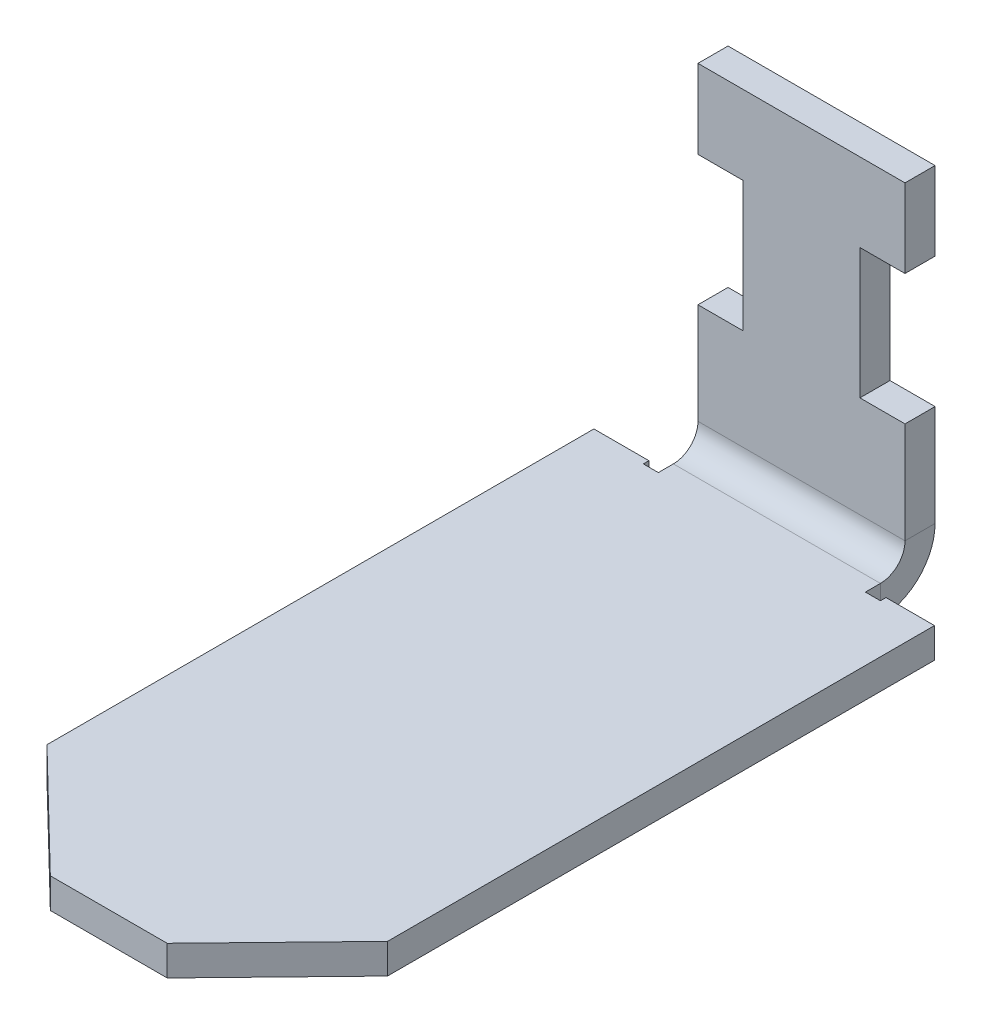
ISO-10303-21;
HEADER;
FILE_DESCRIPTION(('STEP AP214'),'2;1');
FILE_NAME('part.step','',(''),(''),'','','');
FILE_SCHEMA(('AUTOMOTIVE_DESIGN { 1 0 10303 214 1 1 1 1 }'));
ENDSEC;
DATA;
#1=APPLICATION_CONTEXT('core data for automotive mechanical design processes');
#2=APPLICATION_PROTOCOL_DEFINITION('international standard','automotive_design',2000,#1);
#3=PRODUCT_CONTEXT('',#1,'mechanical');
#4=PRODUCT('Part','Part','',(#3));
#5=PRODUCT_RELATED_PRODUCT_CATEGORY('part','',(#4));
#6=PRODUCT_DEFINITION_FORMATION('','',#4);
#7=PRODUCT_DEFINITION_CONTEXT('part definition',#1,'design');
#8=PRODUCT_DEFINITION('design','',#6,#7);
#9=PRODUCT_DEFINITION_SHAPE('','',#8);
#10=(LENGTH_UNIT() NAMED_UNIT(*) SI_UNIT(.MILLI.,.METRE.));
#11=(NAMED_UNIT(*) PLANE_ANGLE_UNIT() SI_UNIT($,.RADIAN.));
#12=(NAMED_UNIT(*) SI_UNIT($,.STERADIAN.) SOLID_ANGLE_UNIT());
#13=UNCERTAINTY_MEASURE_WITH_UNIT(LENGTH_MEASURE(1.E-05),#10,'distance_accuracy_value','');
#14=(GEOMETRIC_REPRESENTATION_CONTEXT(3) GLOBAL_UNCERTAINTY_ASSIGNED_CONTEXT((#13)) GLOBAL_UNIT_ASSIGNED_CONTEXT((#10,
#11,#12)) REPRESENTATION_CONTEXT('',''));
#15=CARTESIAN_POINT('',(0.,0.,0.));
#16=DIRECTION('',(0.,0.,1.));
#17=DIRECTION('',(1.,0.,0.));
#18=AXIS2_PLACEMENT_3D('',#15,#16,#17);
#19=CARTESIAN_POINT('',(-3.00317944668726,10.02,-10.825));
#20=DIRECTION('',(1.,0.,0.));
#21=DIRECTION('',(0.,0.,-1.));
#22=AXIS2_PLACEMENT_3D('',#19,#20,#21);
#23=PLANE('',#22);
#24=DIRECTION('',(0.,0.,1.));
#25=VECTOR('',#24,1.);
#26=CARTESIAN_POINT('',(-3.00317944668726,7.65880268385961,-10.825));
#27=LINE('',#26,#25);
#28=CARTESIAN_POINT('',(-3.00317944668726,7.65880268385961,-10.825));
#29=VERTEX_POINT('',#28);
#30=CARTESIAN_POINT('',(-3.00317944668726,7.65880268385961,-9.925));
#31=VERTEX_POINT('',#30);
#32=EDGE_CURVE('E269',#29,#31,#27,.T.);
#33=ORIENTED_EDGE('',*,*,#32,.T.);
#34=DIRECTION('',(0.,-1.,0.));
#35=VECTOR('',#34,1.);
#36=CARTESIAN_POINT('',(-3.00317944668726,10.02,-9.92500000000003));
#37=LINE('',#36,#35);
#38=CARTESIAN_POINT('',(-3.00317944668726,10.02,-9.92500000000003));
#39=VERTEX_POINT('',#38);
#40=EDGE_CURVE('E324',#31,#39,#37,.F.);
#41=ORIENTED_EDGE('',*,*,#40,.T.);
#42=DIRECTION('',(0.,0.,1.));
#43=VECTOR('',#42,1.);
#44=CARTESIAN_POINT('',(-3.00317944668726,10.02,-10.825));
#45=LINE('',#44,#43);
#46=CARTESIAN_POINT('',(-3.00317944668726,10.02,-10.825));
#47=VERTEX_POINT('',#46);
#48=EDGE_CURVE('E300',#47,#39,#45,.T.);
#49=ORIENTED_EDGE('',*,*,#48,.F.);
#50=DIRECTION('',(0.,1.,0.));
#51=VECTOR('',#50,1.);
#52=CARTESIAN_POINT('',(-3.00317944668726,0.,-10.825));
#53=LINE('',#52,#51);
#54=EDGE_CURVE('E311',#29,#47,#53,.T.);
#55=ORIENTED_EDGE('',*,*,#54,.F.);
#56=EDGE_LOOP('',(#33,#41,#49,#55));
#57=FACE_BOUND('',#56,.T.);
#58=ADVANCED_FACE('F65',(#57),#23,.F.);
#59=CARTESIAN_POINT('',(3.19682055331274,0.,-10.825));
#60=DIRECTION('',(-1.,0.,0.));
#61=DIRECTION('',(0.,0.,1.));
#62=AXIS2_PLACEMENT_3D('',#59,#60,#61);
#63=PLANE('',#62);
#64=DIRECTION('',(0.,0.,1.));
#65=VECTOR('',#64,1.);
#66=CARTESIAN_POINT('',(3.19682055331274,3.76868388204292,-10.825));
#67=LINE('',#66,#65);
#68=CARTESIAN_POINT('',(3.19682055331274,3.76868388204292,-10.825));
#69=VERTEX_POINT('',#68);
#70=CARTESIAN_POINT('',(3.19682055331274,3.76868388204292,-9.925));
#71=VERTEX_POINT('',#70);
#72=EDGE_CURVE('E278',#69,#71,#67,.T.);
#73=ORIENTED_EDGE('',*,*,#72,.T.);
#74=DIRECTION('',(0.,1.,0.));
#75=VECTOR('',#74,1.);
#76=CARTESIAN_POINT('',(3.19682055331274,0.,-9.925));
#77=LINE('',#76,#75);
#78=CARTESIAN_POINT('',(3.19682055331274,0.736599999999989,-9.925));
#79=VERTEX_POINT('',#78);
#80=EDGE_CURVE('E314',#71,#79,#77,.F.);
#81=ORIENTED_EDGE('',*,*,#80,.T.);
#82=DIRECTION('',(0.,0.,1.));
#83=VECTOR('',#82,1.);
#84=CARTESIAN_POINT('',(3.19682055331274,0.736600000000003,-10.825));
#85=LINE('',#84,#83);
#86=CARTESIAN_POINT('',(3.19682055331274,0.736599999999986,-10.825));
#87=VERTEX_POINT('',#86);
#88=EDGE_CURVE('E268',#79,#87,#85,.F.);
#89=ORIENTED_EDGE('',*,*,#88,.T.);
#90=DIRECTION('',(0.,-1.,0.));
#91=VECTOR('',#90,1.);
#92=CARTESIAN_POINT('',(3.19682055331274,0.,-10.825));
#93=LINE('',#92,#91);
#94=EDGE_CURVE('E310',#69,#87,#93,.T.);
#95=ORIENTED_EDGE('',*,*,#94,.F.);
#96=EDGE_LOOP('',(#73,#81,#89,#95));
#97=FACE_BOUND('',#96,.T.);
#98=ADVANCED_FACE('F516',(#97),#63,.F.);
#99=CARTESIAN_POINT('',(0.,0.,-10.825));
#100=DIRECTION('',(0.,0.,1.));
#101=DIRECTION('',(0.,-1.,0.));
#102=AXIS2_PLACEMENT_3D('',#99,#100,#101);
#103=PLANE('',#102);
#104=CARTESIAN_POINT('',(-3.00317944668726,0.736600000000003,-10.825));
#105=VERTEX_POINT('',#104);
#106=CARTESIAN_POINT('',(-3.00317944668726,3.75880268385961,-10.825));
#107=VERTEX_POINT('',#106);
#108=EDGE_CURVE('E259',#105,#107,#53,.T.);
#109=ORIENTED_EDGE('',*,*,#108,.T.);
#110=DIRECTION('',(1.,0.,0.));
#111=VECTOR('',#110,1.);
#112=CARTESIAN_POINT('',(-3.00317944668726,3.75880268385961,-10.825));
#113=LINE('',#112,#111);
#114=CARTESIAN_POINT('',(-1.65317944668726,3.75880268385961,-10.825));
#115=VERTEX_POINT('',#114);
#116=EDGE_CURVE('E250',#107,#115,#113,.T.);
#117=ORIENTED_EDGE('',*,*,#116,.T.);
#118=DIRECTION('',(0.,-1.,0.));
#119=VECTOR('',#118,1.);
#120=CARTESIAN_POINT('',(-1.65317944668726,7.65880268385961,-10.825));
#121=LINE('',#120,#119);
#122=CARTESIAN_POINT('',(-1.65317944668726,7.65880268385961,-10.825));
#123=VERTEX_POINT('',#122);
#124=EDGE_CURVE('E240',#123,#115,#121,.T.);
#125=ORIENTED_EDGE('',*,*,#124,.F.);
#126=DIRECTION('',(1.,0.,0.));
#127=VECTOR('',#126,1.);
#128=CARTESIAN_POINT('',(-3.00317944668726,7.65880268385961,-10.825));
#129=LINE('',#128,#127);
#130=EDGE_CURVE('E246',#29,#123,#129,.T.);
#131=ORIENTED_EDGE('',*,*,#130,.F.);
#132=ORIENTED_EDGE('',*,*,#54,.T.);
#133=DIRECTION('',(1.,0.,0.));
#134=VECTOR('',#133,1.);
#135=CARTESIAN_POINT('',(0.,10.02,-10.825));
#136=LINE('',#135,#134);
#137=CARTESIAN_POINT('',(3.19682055331274,10.02,-10.825));
#138=VERTEX_POINT('',#137);
#139=EDGE_CURVE('E308',#47,#138,#136,.T.);
#140=ORIENTED_EDGE('',*,*,#139,.T.);
#141=CARTESIAN_POINT('',(3.19682055331274,7.66868388204292,-10.825));
#142=VERTEX_POINT('',#141);
#143=EDGE_CURVE('E302',#138,#142,#93,.T.);
#144=ORIENTED_EDGE('',*,*,#143,.T.);
#145=DIRECTION('',(-1.,0.,0.));
#146=VECTOR('',#145,1.);
#147=CARTESIAN_POINT('',(3.19682055331274,7.66868388204292,-10.825));
#148=LINE('',#147,#146);
#149=CARTESIAN_POINT('',(1.84682055331274,7.66868388204292,-10.825));
#150=VERTEX_POINT('',#149);
#151=EDGE_CURVE('E285',#142,#150,#148,.T.);
#152=ORIENTED_EDGE('',*,*,#151,.T.);
#153=DIRECTION('',(0.,-1.,0.));
#154=VECTOR('',#153,1.);
#155=CARTESIAN_POINT('',(1.84682055331274,7.66868388204292,-10.825));
#156=LINE('',#155,#154);
#157=CARTESIAN_POINT('',(1.84682055331274,3.76868388204292,-10.825));
#158=VERTEX_POINT('',#157);
#159=EDGE_CURVE('E291',#150,#158,#156,.T.);
#160=ORIENTED_EDGE('',*,*,#159,.T.);
#161=DIRECTION('',(-1.,0.,0.));
#162=VECTOR('',#161,1.);
#163=CARTESIAN_POINT('',(3.19682055331274,3.76868388204292,-10.825));
#164=LINE('',#163,#162);
#165=EDGE_CURVE('E288',#69,#158,#164,.T.);
#166=ORIENTED_EDGE('',*,*,#165,.F.);
#167=ORIENTED_EDGE('',*,*,#94,.T.);
#168=DIRECTION('',(-1.,0.,0.));
#169=VECTOR('',#168,1.);
#170=CARTESIAN_POINT('',(3.19682055331274,0.736600000000003,-10.825));
#171=LINE('',#170,#169);
#172=EDGE_CURVE('E321',#105,#87,#171,.F.);
#173=ORIENTED_EDGE('',*,*,#172,.F.);
#174=EDGE_LOOP('',(#109,#117,#125,#131,#132,#140,#144,#152,#160,#166,#167,#173));
#175=FACE_BOUND('',#174,.T.);
#176=ADVANCED_FACE('F254',(#175),#103,.F.);
#177=CARTESIAN_POINT('',(0.,0.,-9.925));
#178=DIRECTION('',(0.,0.,1.));
#179=DIRECTION('',(0.,-1.,0.));
#180=AXIS2_PLACEMENT_3D('',#177,#178,#179);
#181=PLANE('',#180);
#182=DIRECTION('',(1.,0.,0.));
#183=VECTOR('',#182,1.);
#184=CARTESIAN_POINT('',(-3.00317944668726,3.75880268385961,-9.925));
#185=LINE('',#184,#183);
#186=CARTESIAN_POINT('',(-3.00317944668726,3.75880268385961,-9.925));
#187=VERTEX_POINT('',#186);
#188=CARTESIAN_POINT('',(-1.65317944668726,3.75880268385961,-9.92500000000001));
#189=VERTEX_POINT('',#188);
#190=EDGE_CURVE('E76',#187,#189,#185,.T.);
#191=ORIENTED_EDGE('',*,*,#190,.F.);
#192=CARTESIAN_POINT('',(-3.00317944668726,0.736599999999989,-9.925));
#193=VERTEX_POINT('',#192);
#194=EDGE_CURVE('E319',#193,#187,#37,.F.);
#195=ORIENTED_EDGE('',*,*,#194,.F.);
#196=DIRECTION('',(-1.,0.,0.));
#197=VECTOR('',#196,1.);
#198=CARTESIAN_POINT('',(3.19682055331274,0.736599999999997,-9.925));
#199=LINE('',#198,#197);
#200=EDGE_CURVE('E327',#79,#193,#199,.T.);
#201=ORIENTED_EDGE('',*,*,#200,.F.);
#202=ORIENTED_EDGE('',*,*,#80,.F.);
#203=DIRECTION('',(-1.,0.,0.));
#204=VECTOR('',#203,1.);
#205=CARTESIAN_POINT('',(3.19682055331274,3.76868388204292,-9.925));
#206=LINE('',#205,#204);
#207=CARTESIAN_POINT('',(1.84682055331274,3.76868388204292,-9.925));
#208=VERTEX_POINT('',#207);
#209=EDGE_CURVE('E261',#71,#208,#206,.T.);
#210=ORIENTED_EDGE('',*,*,#209,.T.);
#211=DIRECTION('',(0.,-1.,0.));
#212=VECTOR('',#211,1.);
#213=CARTESIAN_POINT('',(1.84682055331274,7.66868388204292,-9.925));
#214=LINE('',#213,#212);
#215=CARTESIAN_POINT('',(1.84682055331274,7.66868388204292,-9.925));
#216=VERTEX_POINT('',#215);
#217=EDGE_CURVE('E284',#216,#208,#214,.T.);
#218=ORIENTED_EDGE('',*,*,#217,.F.);
#219=DIRECTION('',(-1.,0.,0.));
#220=VECTOR('',#219,1.);
#221=CARTESIAN_POINT('',(3.19682055331274,7.66868388204292,-9.925));
#222=LINE('',#221,#220);
#223=CARTESIAN_POINT('',(3.19682055331274,7.66868388204292,-9.92500000000002));
#224=VERTEX_POINT('',#223);
#225=EDGE_CURVE('E282',#224,#216,#222,.T.);
#226=ORIENTED_EDGE('',*,*,#225,.F.);
#227=CARTESIAN_POINT('',(3.19682055331274,10.02,-9.92500000000003));
#228=VERTEX_POINT('',#227);
#229=EDGE_CURVE('E315',#228,#224,#77,.F.);
#230=ORIENTED_EDGE('',*,*,#229,.F.);
#231=DIRECTION('',(-1.,0.,0.));
#232=VECTOR('',#231,1.);
#233=CARTESIAN_POINT('',(3.19682055331274,10.02,-9.92500000000003));
#234=LINE('',#233,#232);
#235=EDGE_CURVE('E317',#39,#228,#234,.F.);
#236=ORIENTED_EDGE('',*,*,#235,.F.);
#237=ORIENTED_EDGE('',*,*,#40,.F.);
#238=DIRECTION('',(1.,0.,0.));
#239=VECTOR('',#238,1.);
#240=CARTESIAN_POINT('',(-3.00317944668726,7.65880268385961,-9.925));
#241=LINE('',#240,#239);
#242=CARTESIAN_POINT('',(-1.65317944668726,7.65880268385961,-9.925));
#243=VERTEX_POINT('',#242);
#244=EDGE_CURVE('E256',#31,#243,#241,.T.);
#245=ORIENTED_EDGE('',*,*,#244,.T.);
#246=DIRECTION('',(0.,-1.,0.));
#247=VECTOR('',#246,1.);
#248=CARTESIAN_POINT('',(-1.65317944668726,7.65880268385961,-9.925));
#249=LINE('',#248,#247);
#250=EDGE_CURVE('E257',#243,#189,#249,.T.);
#251=ORIENTED_EDGE('',*,*,#250,.T.);
#252=EDGE_LOOP('',(#191,#195,#201,#202,#210,#218,#226,#230,#236,#237,#245,#251));
#253=FACE_BOUND('',#252,.T.);
#254=ADVANCED_FACE('F495',(#253),#181,.T.);
#255=CARTESIAN_POINT('',(0.,-0.9,0.));
#256=DIRECTION('',(0.,1.,0.));
#257=DIRECTION('',(0.,0.,1.));
#258=AXIS2_PLACEMENT_3D('',#255,#256,#257);
#259=PLANE('',#258);
#260=DIRECTION('',(0.,0.,-1.));
#261=VECTOR('',#260,1.);
#262=CARTESIAN_POINT('',(-3.45317944668726,-0.9,0.));
#263=LINE('',#262,#261);
#264=CARTESIAN_POINT('',(-3.45317944668726,-0.9,-8.7384));
#265=VERTEX_POINT('',#264);
#266=CARTESIAN_POINT('',(-3.45317944668726,-0.9,-8.905));
#267=VERTEX_POINT('',#266);
#268=EDGE_CURVE('E357',#265,#267,#263,.T.);
#269=ORIENTED_EDGE('',*,*,#268,.F.);
#270=DIRECTION('',(-1.,0.,0.));
#271=VECTOR('',#270,1.);
#272=CARTESIAN_POINT('',(0.,-0.9,-8.7384));
#273=LINE('',#272,#271);
#274=CARTESIAN_POINT('',(-3.00317944668726,-0.9,-8.7384));
#275=VERTEX_POINT('',#274);
#276=EDGE_CURVE('E383',#275,#265,#273,.T.);
#277=ORIENTED_EDGE('',*,*,#276,.F.);
#278=DIRECTION('',(0.,0.,1.));
#279=VECTOR('',#278,1.);
#280=CARTESIAN_POINT('',(-3.00317944668726,-0.9,0.));
#281=LINE('',#280,#279);
#282=CARTESIAN_POINT('',(-3.00317944668726,-0.900000000000009,-9.1884));
#283=VERTEX_POINT('',#282);
#284=EDGE_CURVE('E407',#283,#275,#281,.T.);
#285=ORIENTED_EDGE('',*,*,#284,.F.);
#286=DIRECTION('',(-1.,0.,0.));
#287=VECTOR('',#286,1.);
#288=CARTESIAN_POINT('',(-3.00317944668726,-0.900000000000009,-9.1884));
#289=LINE('',#288,#287);
#290=CARTESIAN_POINT('',(3.19682055331274,-0.9,-9.1884));
#291=VERTEX_POINT('',#290);
#292=EDGE_CURVE('E335',#283,#291,#289,.F.);
#293=ORIENTED_EDGE('',*,*,#292,.T.);
#294=DIRECTION('',(0.,0.,1.));
#295=VECTOR('',#294,1.);
#296=CARTESIAN_POINT('',(3.19682055331274,-0.9,0.));
#297=LINE('',#296,#295);
#298=CARTESIAN_POINT('',(3.19682055331274,-0.9,-8.7384));
#299=VERTEX_POINT('',#298);
#300=EDGE_CURVE('E423',#291,#299,#297,.T.);
#301=ORIENTED_EDGE('',*,*,#300,.T.);
#302=DIRECTION('',(-1.,0.,0.));
#303=VECTOR('',#302,1.);
#304=CARTESIAN_POINT('',(0.,-0.9,-8.7384));
#305=LINE('',#304,#303);
#306=CARTESIAN_POINT('',(3.64682055331274,-0.9,-8.7384));
#307=VERTEX_POINT('',#306);
#308=EDGE_CURVE('E385',#307,#299,#305,.T.);
#309=ORIENTED_EDGE('',*,*,#308,.F.);
#310=DIRECTION('',(0.,0.,1.));
#311=VECTOR('',#310,1.);
#312=CARTESIAN_POINT('',(3.64682055331274,-0.9,0.));
#313=LINE('',#312,#311);
#314=CARTESIAN_POINT('',(3.64682055331274,-0.9,-8.905));
#315=VERTEX_POINT('',#314);
#316=EDGE_CURVE('E378',#315,#307,#313,.T.);
#317=ORIENTED_EDGE('',*,*,#316,.F.);
#318=DIRECTION('',(-1.,0.,0.));
#319=VECTOR('',#318,1.);
#320=CARTESIAN_POINT('',(0.,-0.9,-8.905));
#321=LINE('',#320,#319);
#322=CARTESIAN_POINT('',(5.1,-0.9,-8.905));
#323=VERTEX_POINT('',#322);
#324=EDGE_CURVE('E421',#323,#315,#321,.T.);
#325=ORIENTED_EDGE('',*,*,#324,.F.);
#326=DIRECTION('',(0.,0.,-1.));
#327=VECTOR('',#326,1.);
#328=CARTESIAN_POINT('',(5.1,-0.9,-10.825));
#329=LINE('',#328,#327);
#330=CARTESIAN_POINT('',(5.1,-0.9,7.475));
#331=VERTEX_POINT('',#330);
#332=EDGE_CURVE('E435',#331,#323,#329,.T.);
#333=ORIENTED_EDGE('',*,*,#332,.F.);
#334=DIRECTION('',(0.69615869955734,0.,-0.717887919546383));
#335=VECTOR('',#334,1.);
#336=CARTESIAN_POINT('',(6.36408693738875,-0.9,6.17145708344262));
#337=LINE('',#336,#335);
#338=CARTESIAN_POINT('',(1.85139867934996,-0.9,10.825));
#339=VERTEX_POINT('',#338);
#340=EDGE_CURVE('E390',#339,#331,#337,.T.);
#341=ORIENTED_EDGE('',*,*,#340,.F.);
#342=DIRECTION('',(1.,0.,0.));
#343=VECTOR('',#342,1.);
#344=CARTESIAN_POINT('',(-5.1,-0.9,10.825));
#345=LINE('',#344,#343);
#346=CARTESIAN_POINT('',(-1.64860132065004,-0.9,10.825));
#347=VERTEX_POINT('',#346);
#348=EDGE_CURVE('E438',#347,#339,#345,.T.);
#349=ORIENTED_EDGE('',*,*,#348,.F.);
#350=DIRECTION('',(0.717568945196471,0.,0.696487479348785));
#351=VECTOR('',#350,1.);
#352=CARTESIAN_POINT('',(-6.20982247493104,-0.9,6.39778301163423));
#353=LINE('',#352,#351);
#354=CARTESIAN_POINT('',(-5.1,-0.9,7.475));
#355=VERTEX_POINT('',#354);
#356=EDGE_CURVE('E399',#355,#347,#353,.T.);
#357=ORIENTED_EDGE('',*,*,#356,.F.);
#358=DIRECTION('',(0.,0.,1.));
#359=VECTOR('',#358,1.);
#360=CARTESIAN_POINT('',(-5.1,-0.9,-10.825));
#361=LINE('',#360,#359);
#362=CARTESIAN_POINT('',(-5.1,-0.9,-8.905));
#363=VERTEX_POINT('',#362);
#364=EDGE_CURVE('E432',#363,#355,#361,.T.);
#365=ORIENTED_EDGE('',*,*,#364,.F.);
#366=DIRECTION('',(-1.,0.,0.));
#367=VECTOR('',#366,1.);
#368=CARTESIAN_POINT('',(0.,-0.9,-8.905));
#369=LINE('',#368,#367);
#370=EDGE_CURVE('E410',#267,#363,#369,.T.);
#371=ORIENTED_EDGE('',*,*,#370,.F.);
#372=EDGE_LOOP('',(#269,#277,#285,#293,#301,#309,#317,#325,#333,#341,#349,#357,#365,#371));
#373=FACE_BOUND('',#372,.T.);
#374=ADVANCED_FACE('F459',(#373),#259,.F.);
#375=CARTESIAN_POINT('',(0.,0.,0.));
#376=DIRECTION('',(0.,1.,0.));
#377=DIRECTION('',(0.,0.,1.));
#378=AXIS2_PLACEMENT_3D('',#375,#376,#377);
#379=PLANE('',#378);
#380=DIRECTION('',(1.,0.,0.));
#381=VECTOR('',#380,1.);
#382=CARTESIAN_POINT('',(-3.45317944668726,0.,-8.7384));
#383=LINE('',#382,#381);
#384=CARTESIAN_POINT('',(-3.45317944668726,0.,-8.7384));
#385=VERTEX_POINT('',#384);
#386=CARTESIAN_POINT('',(-3.00317944668726,0.,-8.7384));
#387=VERTEX_POINT('',#386);
#388=EDGE_CURVE('E356',#385,#387,#383,.T.);
#389=ORIENTED_EDGE('',*,*,#388,.F.);
#390=DIRECTION('',(0.,0.,1.));
#391=VECTOR('',#390,1.);
#392=CARTESIAN_POINT('',(-3.45317944668726,0.,-10.825));
#393=LINE('',#392,#391);
#394=CARTESIAN_POINT('',(-3.45317944668726,0.,-8.905));
#395=VERTEX_POINT('',#394);
#396=EDGE_CURVE('E351',#395,#385,#393,.T.);
#397=ORIENTED_EDGE('',*,*,#396,.F.);
#398=DIRECTION('',(-1.,0.,0.));
#399=VECTOR('',#398,1.);
#400=CARTESIAN_POINT('',(0.,0.,-8.905));
#401=LINE('',#400,#399);
#402=CARTESIAN_POINT('',(-5.1,0.,-8.905));
#403=VERTEX_POINT('',#402);
#404=EDGE_CURVE('E413',#395,#403,#401,.T.);
#405=ORIENTED_EDGE('',*,*,#404,.T.);
#406=DIRECTION('',(0.,0.,1.));
#407=VECTOR('',#406,1.);
#408=CARTESIAN_POINT('',(-5.1,0.,-10.825));
#409=LINE('',#408,#407);
#410=CARTESIAN_POINT('',(-5.1,0.,7.475));
#411=VERTEX_POINT('',#410);
#412=EDGE_CURVE('E445',#403,#411,#409,.T.);
#413=ORIENTED_EDGE('',*,*,#412,.T.);
#414=DIRECTION('',(0.717568945196471,0.,0.696487479348785));
#415=VECTOR('',#414,1.);
#416=CARTESIAN_POINT('',(-6.20982247493104,0.,6.39778301163423));
#417=LINE('',#416,#415);
#418=CARTESIAN_POINT('',(-1.64860132065004,0.,10.825));
#419=VERTEX_POINT('',#418);
#420=EDGE_CURVE('E386',#411,#419,#417,.T.);
#421=ORIENTED_EDGE('',*,*,#420,.T.);
#422=DIRECTION('',(1.,0.,0.));
#423=VECTOR('',#422,1.);
#424=CARTESIAN_POINT('',(-5.1,0.,10.825));
#425=LINE('',#424,#423);
#426=CARTESIAN_POINT('',(1.85139867934996,0.,10.825));
#427=VERTEX_POINT('',#426);
#428=EDGE_CURVE('E434',#419,#427,#425,.T.);
#429=ORIENTED_EDGE('',*,*,#428,.T.);
#430=DIRECTION('',(0.69615869955734,0.,-0.717887919546383));
#431=VECTOR('',#430,1.);
#432=CARTESIAN_POINT('',(6.36408693738875,0.,6.17145708344262));
#433=LINE('',#432,#431);
#434=CARTESIAN_POINT('',(5.1,0.,7.475));
#435=VERTEX_POINT('',#434);
#436=EDGE_CURVE('E393',#427,#435,#433,.T.);
#437=ORIENTED_EDGE('',*,*,#436,.T.);
#438=DIRECTION('',(0.,0.,-1.));
#439=VECTOR('',#438,1.);
#440=CARTESIAN_POINT('',(5.1,0.,-10.825));
#441=LINE('',#440,#439);
#442=CARTESIAN_POINT('',(5.1,0.,-8.905));
#443=VERTEX_POINT('',#442);
#444=EDGE_CURVE('E416',#435,#443,#441,.T.);
#445=ORIENTED_EDGE('',*,*,#444,.T.);
#446=DIRECTION('',(-1.,0.,0.));
#447=VECTOR('',#446,1.);
#448=CARTESIAN_POINT('',(0.,0.,-8.905));
#449=LINE('',#448,#447);
#450=CARTESIAN_POINT('',(3.64682055331274,0.,-8.905));
#451=VERTEX_POINT('',#450);
#452=EDGE_CURVE('E425',#443,#451,#449,.T.);
#453=ORIENTED_EDGE('',*,*,#452,.T.);
#454=DIRECTION('',(0.,0.,-1.));
#455=VECTOR('',#454,1.);
#456=CARTESIAN_POINT('',(3.64682055331274,0.,-8.7384));
#457=LINE('',#456,#455);
#458=CARTESIAN_POINT('',(3.64682055331274,0.,-8.7384));
#459=VERTEX_POINT('',#458);
#460=EDGE_CURVE('E370',#459,#451,#457,.T.);
#461=ORIENTED_EDGE('',*,*,#460,.F.);
#462=DIRECTION('',(1.,0.,0.));
#463=VECTOR('',#462,1.);
#464=CARTESIAN_POINT('',(3.19682055331274,0.,-8.7384));
#465=LINE('',#464,#463);
#466=CARTESIAN_POINT('',(3.19682055331274,0.,-8.7384));
#467=VERTEX_POINT('',#466);
#468=EDGE_CURVE('E365',#467,#459,#465,.T.);
#469=ORIENTED_EDGE('',*,*,#468,.F.);
#470=DIRECTION('',(0.,0.,1.));
#471=VECTOR('',#470,1.);
#472=CARTESIAN_POINT('',(3.19682055331274,0.,0.));
#473=LINE('',#472,#471);
#474=CARTESIAN_POINT('',(3.19682055331274,0.,-9.1884));
#475=VERTEX_POINT('',#474);
#476=EDGE_CURVE('E400',#475,#467,#473,.T.);
#477=ORIENTED_EDGE('',*,*,#476,.F.);
#478=DIRECTION('',(-1.,0.,0.));
#479=VECTOR('',#478,1.);
#480=CARTESIAN_POINT('',(-3.00317944668726,0.,-9.1884));
#481=LINE('',#480,#479);
#482=CARTESIAN_POINT('',(-3.00317944668726,0.,-9.1884));
#483=VERTEX_POINT('',#482);
#484=EDGE_CURVE('E343',#483,#475,#481,.F.);
#485=ORIENTED_EDGE('',*,*,#484,.F.);
#486=DIRECTION('',(0.,0.,1.));
#487=VECTOR('',#486,1.);
#488=CARTESIAN_POINT('',(-3.00317944668726,0.,0.));
#489=LINE('',#488,#487);
#490=EDGE_CURVE('E411',#483,#387,#489,.T.);
#491=ORIENTED_EDGE('',*,*,#490,.T.);
#492=EDGE_LOOP('',(#389,#397,#405,#413,#421,#429,#437,#445,#453,#461,#469,#477,#485,#491));
#493=FACE_BOUND('',#492,.T.);
#494=ADVANCED_FACE('F467',(#493),#379,.T.);
#495=CARTESIAN_POINT('',(0.,-0.9,-8.905));
#496=DIRECTION('',(0.,0.,-1.));
#497=DIRECTION('',(-1.,0.,0.));
#498=AXIS2_PLACEMENT_3D('',#495,#496,#497);
#499=PLANE('',#498);
#500=ORIENTED_EDGE('',*,*,#324,.T.);
#501=DIRECTION('',(0.,1.,0.));
#502=VECTOR('',#501,1.);
#503=CARTESIAN_POINT('',(3.64682055331274,-0.9,-8.905));
#504=LINE('',#503,#502);
#505=EDGE_CURVE('E13',#315,#451,#504,.T.);
#506=ORIENTED_EDGE('',*,*,#505,.T.);
#507=ORIENTED_EDGE('',*,*,#452,.F.);
#508=DIRECTION('',(0.,1.,0.));
#509=VECTOR('',#508,1.);
#510=CARTESIAN_POINT('',(5.1,-0.9,-8.905));
#511=LINE('',#510,#509);
#512=EDGE_CURVE('E418',#323,#443,#511,.T.);
#513=ORIENTED_EDGE('',*,*,#512,.F.);
#514=EDGE_LOOP('',(#500,#506,#507,#513));
#515=FACE_BOUND('',#514,.T.);
#516=ADVANCED_FACE('F585',(#515),#499,.T.);
#517=CARTESIAN_POINT('',(3.19682055331274,-0.9,0.));
#518=DIRECTION('',(-1.,0.,0.));
#519=DIRECTION('',(0.,0.,1.));
#520=AXIS2_PLACEMENT_3D('',#517,#518,#519);
#521=PLANE('',#520);
#522=DIRECTION('',(0.,-1.,0.));
#523=VECTOR('',#522,1.);
#524=CARTESIAN_POINT('',(3.19682055331274,0.,-9.1884));
#525=LINE('',#524,#523);
#526=EDGE_CURVE('E348',#475,#291,#525,.T.);
#527=ORIENTED_EDGE('',*,*,#526,.F.);
#528=ORIENTED_EDGE('',*,*,#476,.T.);
#529=DIRECTION('',(0.,-1.,0.));
#530=VECTOR('',#529,1.);
#531=CARTESIAN_POINT('',(3.19682055331274,0.,-8.7384));
#532=LINE('',#531,#530);
#533=EDGE_CURVE('E366',#467,#299,#532,.T.);
#534=ORIENTED_EDGE('',*,*,#533,.T.);
#535=ORIENTED_EDGE('',*,*,#300,.F.);
#536=EDGE_LOOP('',(#527,#528,#534,#535));
#537=FACE_BOUND('',#536,.T.);
#538=ADVANCED_FACE('F581',(#537),#521,.F.);
#539=CARTESIAN_POINT('',(0.,-0.9,-8.905));
#540=DIRECTION('',(0.,0.,-1.));
#541=DIRECTION('',(-1.,0.,0.));
#542=AXIS2_PLACEMENT_3D('',#539,#540,#541);
#543=PLANE('',#542);
#544=ORIENTED_EDGE('',*,*,#404,.F.);
#545=DIRECTION('',(0.,-1.,0.));
#546=VECTOR('',#545,1.);
#547=CARTESIAN_POINT('',(-3.45317944668726,-0.9,-8.905));
#548=LINE('',#547,#546);
#549=EDGE_CURVE('E71',#395,#267,#548,.T.);
#550=ORIENTED_EDGE('',*,*,#549,.T.);
#551=ORIENTED_EDGE('',*,*,#370,.T.);
#552=DIRECTION('',(0.,1.,0.));
#553=VECTOR('',#552,1.);
#554=CARTESIAN_POINT('',(-5.1,-0.9,-8.905));
#555=LINE('',#554,#553);
#556=EDGE_CURVE('E412',#363,#403,#555,.T.);
#557=ORIENTED_EDGE('',*,*,#556,.T.);
#558=EDGE_LOOP('',(#544,#550,#551,#557));
#559=FACE_BOUND('',#558,.T.);
#560=ADVANCED_FACE('F448',(#559),#543,.T.);
#561=CARTESIAN_POINT('',(-3.00317944668726,-0.9,0.));
#562=DIRECTION('',(-1.,0.,0.));
#563=DIRECTION('',(0.,0.,1.));
#564=AXIS2_PLACEMENT_3D('',#561,#562,#563);
#565=PLANE('',#564);
#566=ORIENTED_EDGE('',*,*,#490,.F.);
#567=DIRECTION('',(0.,-1.,0.));
#568=VECTOR('',#567,1.);
#569=CARTESIAN_POINT('',(-3.00317944668726,0.,-9.1884));
#570=LINE('',#569,#568);
#571=EDGE_CURVE('E336',#483,#283,#570,.T.);
#572=ORIENTED_EDGE('',*,*,#571,.T.);
#573=ORIENTED_EDGE('',*,*,#284,.T.);
#574=DIRECTION('',(0.,-1.,0.));
#575=VECTOR('',#574,1.);
#576=CARTESIAN_POINT('',(-3.00317944668726,0.,-8.7384));
#577=LINE('',#576,#575);
#578=EDGE_CURVE('E362',#387,#275,#577,.T.);
#579=ORIENTED_EDGE('',*,*,#578,.F.);
#580=EDGE_LOOP('',(#566,#572,#573,#579));
#581=FACE_BOUND('',#580,.T.);
#582=ADVANCED_FACE('F477',(#581),#565,.T.);
#583=CARTESIAN_POINT('',(5.1,-0.9,-10.825));
#584=DIRECTION('',(1.,0.,0.));
#585=DIRECTION('',(0.,0.,-1.));
#586=AXIS2_PLACEMENT_3D('',#583,#584,#585);
#587=PLANE('',#586);
#588=ORIENTED_EDGE('',*,*,#444,.F.);
#589=DIRECTION('',(0.,1.,0.));
#590=VECTOR('',#589,1.);
#591=CARTESIAN_POINT('',(5.1,-0.9,7.475));
#592=LINE('',#591,#590);
#593=EDGE_CURVE('E391',#331,#435,#592,.T.);
#594=ORIENTED_EDGE('',*,*,#593,.F.);
#595=ORIENTED_EDGE('',*,*,#332,.T.);
#596=ORIENTED_EDGE('',*,*,#512,.T.);
#597=EDGE_LOOP('',(#588,#594,#595,#596));
#598=FACE_BOUND('',#597,.T.);
#599=ADVANCED_FACE('F62',(#598),#587,.T.);
#600=CARTESIAN_POINT('',(-5.1,-0.9,-10.825));
#601=DIRECTION('',(-1.,0.,0.));
#602=DIRECTION('',(0.,0.,1.));
#603=AXIS2_PLACEMENT_3D('',#600,#601,#602);
#604=PLANE('',#603);
#605=ORIENTED_EDGE('',*,*,#364,.T.);
#606=DIRECTION('',(0.,1.,0.));
#607=VECTOR('',#606,1.);
#608=CARTESIAN_POINT('',(-5.1,-0.9,7.475));
#609=LINE('',#608,#607);
#610=EDGE_CURVE('E405',#355,#411,#609,.T.);
#611=ORIENTED_EDGE('',*,*,#610,.T.);
#612=ORIENTED_EDGE('',*,*,#412,.F.);
#613=ORIENTED_EDGE('',*,*,#556,.F.);
#614=EDGE_LOOP('',(#605,#611,#612,#613));
#615=FACE_BOUND('',#614,.T.);
#616=ADVANCED_FACE('F465',(#615),#604,.T.);
#617=CARTESIAN_POINT('',(-5.1,-0.9,10.825));
#618=DIRECTION('',(0.,0.,1.));
#619=DIRECTION('',(1.,0.,0.));
#620=AXIS2_PLACEMENT_3D('',#617,#618,#619);
#621=PLANE('',#620);
#622=ORIENTED_EDGE('',*,*,#348,.T.);
#623=DIRECTION('',(0.,1.,0.));
#624=VECTOR('',#623,1.);
#625=CARTESIAN_POINT('',(1.85139867934996,-0.9,10.825));
#626=LINE('',#625,#624);
#627=EDGE_CURVE('E387',#339,#427,#626,.T.);
#628=ORIENTED_EDGE('',*,*,#627,.T.);
#629=ORIENTED_EDGE('',*,*,#428,.F.);
#630=DIRECTION('',(0.,1.,0.));
#631=VECTOR('',#630,1.);
#632=CARTESIAN_POINT('',(-1.64860132065004,-0.9,10.825));
#633=LINE('',#632,#631);
#634=EDGE_CURVE('E395',#347,#419,#633,.T.);
#635=ORIENTED_EDGE('',*,*,#634,.F.);
#636=EDGE_LOOP('',(#622,#628,#629,#635));
#637=FACE_BOUND('',#636,.T.);
#638=ADVANCED_FACE('F577',(#637),#621,.T.);
#639=CARTESIAN_POINT('',(-6.20982247493104,-0.9,6.39778301163423));
#640=DIRECTION('',(-0.696487479348785,0.,0.717568945196471));
#641=DIRECTION('',(0.717568945196471,0.,0.696487479348785));
#642=AXIS2_PLACEMENT_3D('',#639,#640,#641);
#643=PLANE('',#642);
#644=ORIENTED_EDGE('',*,*,#420,.F.);
#645=ORIENTED_EDGE('',*,*,#610,.F.);
#646=ORIENTED_EDGE('',*,*,#356,.T.);
#647=ORIENTED_EDGE('',*,*,#634,.T.);
#648=EDGE_LOOP('',(#644,#645,#646,#647));
#649=FACE_BOUND('',#648,.T.);
#650=ADVANCED_FACE('F575',(#649),#643,.T.);
#651=CARTESIAN_POINT('',(6.36408693738875,-0.9,6.17145708344262));
#652=DIRECTION('',(0.717887919546383,0.,0.69615869955734));
#653=DIRECTION('',(0.69615869955734,0.,-0.717887919546383));
#654=AXIS2_PLACEMENT_3D('',#651,#652,#653);
#655=PLANE('',#654);
#656=ORIENTED_EDGE('',*,*,#436,.F.);
#657=ORIENTED_EDGE('',*,*,#627,.F.);
#658=ORIENTED_EDGE('',*,*,#340,.T.);
#659=ORIENTED_EDGE('',*,*,#593,.T.);
#660=EDGE_LOOP('',(#656,#657,#658,#659));
#661=FACE_BOUND('',#660,.T.);
#662=ADVANCED_FACE('F567',(#661),#655,.T.);
#663=CARTESIAN_POINT('',(-3.45317944668726,0.,-10.825));
#664=DIRECTION('',(1.,0.,0.));
#665=DIRECTION('',(0.,0.,-1.));
#666=AXIS2_PLACEMENT_3D('',#663,#664,#665);
#667=PLANE('',#666);
#668=DIRECTION('',(0.,-1.,0.));
#669=VECTOR('',#668,1.);
#670=CARTESIAN_POINT('',(-3.45317944668726,0.,-8.7384));
#671=LINE('',#670,#669);
#672=EDGE_CURVE('E363',#385,#265,#671,.T.);
#673=ORIENTED_EDGE('',*,*,#672,.T.);
#674=ORIENTED_EDGE('',*,*,#268,.T.);
#675=ORIENTED_EDGE('',*,*,#549,.F.);
#676=ORIENTED_EDGE('',*,*,#396,.T.);
#677=EDGE_LOOP('',(#673,#674,#675,#676));
#678=FACE_BOUND('',#677,.T.);
#679=ADVANCED_FACE('F469',(#678),#667,.T.);
#680=CARTESIAN_POINT('',(-3.45317944668726,0.,-8.7384));
#681=DIRECTION('',(0.,0.,-1.));
#682=DIRECTION('',(0.,1.,0.));
#683=AXIS2_PLACEMENT_3D('',#680,#681,#682);
#684=PLANE('',#683);
#685=ORIENTED_EDGE('',*,*,#578,.T.);
#686=ORIENTED_EDGE('',*,*,#276,.T.);
#687=ORIENTED_EDGE('',*,*,#672,.F.);
#688=ORIENTED_EDGE('',*,*,#388,.T.);
#689=EDGE_LOOP('',(#685,#686,#687,#688));
#690=FACE_BOUND('',#689,.T.);
#691=ADVANCED_FACE('F474',(#690),#684,.T.);
#692=CARTESIAN_POINT('',(3.19682055331274,0.,-8.7384));
#693=DIRECTION('',(0.,0.,-1.));
#694=DIRECTION('',(0.,1.,0.));
#695=AXIS2_PLACEMENT_3D('',#692,#693,#694);
#696=PLANE('',#695);
#697=DIRECTION('',(0.,-1.,0.));
#698=VECTOR('',#697,1.);
#699=CARTESIAN_POINT('',(3.64682055331274,0.,-8.7384));
#700=LINE('',#699,#698);
#701=EDGE_CURVE('E354',#459,#307,#700,.T.);
#702=ORIENTED_EDGE('',*,*,#701,.T.);
#703=ORIENTED_EDGE('',*,*,#308,.T.);
#704=ORIENTED_EDGE('',*,*,#533,.F.);
#705=ORIENTED_EDGE('',*,*,#468,.T.);
#706=EDGE_LOOP('',(#702,#703,#704,#705));
#707=FACE_BOUND('',#706,.T.);
#708=ADVANCED_FACE('F557',(#707),#696,.T.);
#709=CARTESIAN_POINT('',(3.64682055331274,0.,-8.7384));
#710=DIRECTION('',(-1.,0.,0.));
#711=DIRECTION('',(0.,0.,1.));
#712=AXIS2_PLACEMENT_3D('',#709,#710,#711);
#713=PLANE('',#712);
#714=ORIENTED_EDGE('',*,*,#505,.F.);
#715=ORIENTED_EDGE('',*,*,#316,.T.);
#716=ORIENTED_EDGE('',*,*,#701,.F.);
#717=ORIENTED_EDGE('',*,*,#460,.T.);
#718=EDGE_LOOP('',(#714,#715,#716,#717));
#719=FACE_BOUND('',#718,.T.);
#720=ADVANCED_FACE('F554',(#719),#713,.T.);
#721=CARTESIAN_POINT('',(3.19682055331274,0.736599999999992,-9.1884));
#722=DIRECTION('',(1.,0.,0.));
#723=DIRECTION('',(0.,0.,-1.));
#724=AXIS2_PLACEMENT_3D('',#721,#722,#723);
#725=PLANE('',#724);
#726=ORIENTED_EDGE('',*,*,#88,.F.);
#727=CARTESIAN_POINT('',(3.19682055331274,0.736599999999992,-9.1884));
#728=DIRECTION('',(-1.,0.,0.));
#729=DIRECTION('',(0.,0.,1.));
#730=AXIS2_PLACEMENT_3D('',#727,#728,#729);
#731=CIRCLE('',#730,0.7366);
#732=EDGE_CURVE('E344',#475,#79,#731,.F.);
#733=ORIENTED_EDGE('',*,*,#732,.F.);
#734=ORIENTED_EDGE('',*,*,#526,.T.);
#735=CARTESIAN_POINT('',(3.19682055331274,0.736599999999992,-9.1884));
#736=DIRECTION('',(-1.,0.,0.));
#737=DIRECTION('',(0.,0.,1.));
#738=AXIS2_PLACEMENT_3D('',#735,#736,#737);
#739=CIRCLE('',#738,1.6366);
#740=EDGE_CURVE('E333',#291,#87,#739,.F.);
#741=ORIENTED_EDGE('',*,*,#740,.T.);
#742=EDGE_LOOP('',(#726,#733,#734,#741));
#743=FACE_BOUND('',#742,.T.);
#744=ADVANCED_FACE('F524',(#743),#725,.T.);
#745=CARTESIAN_POINT('',(-3.00317944668726,0.736599999999992,-9.1884));
#746=DIRECTION('',(1.,0.,0.));
#747=DIRECTION('',(0.,0.,-1.));
#748=AXIS2_PLACEMENT_3D('',#745,#746,#747);
#749=PLANE('',#748);
#750=CARTESIAN_POINT('',(-3.00317944668726,0.736599999999992,-9.1884));
#751=DIRECTION('',(-1.,0.,0.));
#752=DIRECTION('',(0.,0.,1.));
#753=AXIS2_PLACEMENT_3D('',#750,#751,#752);
#754=CIRCLE('',#753,0.7366);
#755=EDGE_CURVE('E297',#193,#483,#754,.T.);
#756=ORIENTED_EDGE('',*,*,#755,.F.);
#757=DIRECTION('',(0.,0.,1.));
#758=VECTOR('',#757,1.);
#759=CARTESIAN_POINT('',(-3.00317944668726,0.736599999999997,-9.925));
#760=LINE('',#759,#758);
#761=EDGE_CURVE('E322',#193,#105,#760,.F.);
#762=ORIENTED_EDGE('',*,*,#761,.T.);
#763=CARTESIAN_POINT('',(-3.00317944668726,0.736599999999992,-9.1884));
#764=DIRECTION('',(-1.,0.,0.));
#765=DIRECTION('',(0.,0.,1.));
#766=AXIS2_PLACEMENT_3D('',#763,#764,#765);
#767=CIRCLE('',#766,1.6366);
#768=EDGE_CURVE('E334',#105,#283,#767,.T.);
#769=ORIENTED_EDGE('',*,*,#768,.T.);
#770=ORIENTED_EDGE('',*,*,#571,.F.);
#771=EDGE_LOOP('',(#756,#762,#769,#770));
#772=FACE_BOUND('',#771,.T.);
#773=ADVANCED_FACE('F485',(#772),#749,.F.);
#774=CARTESIAN_POINT('',(-3.00317944668726,0.736599999999992,-9.1884));
#775=DIRECTION('',(-1.,0.,0.));
#776=DIRECTION('',(0.,0.,-1.));
#777=AXIS2_PLACEMENT_3D('',#774,#775,#776);
#778=CYLINDRICAL_SURFACE('',#777,1.6366);
#779=ORIENTED_EDGE('',*,*,#292,.F.);
#780=ORIENTED_EDGE('',*,*,#768,.F.);
#781=ORIENTED_EDGE('',*,*,#172,.T.);
#782=ORIENTED_EDGE('',*,*,#740,.F.);
#783=EDGE_LOOP('',(#779,#780,#781,#782));
#784=FACE_BOUND('',#783,.T.);
#785=ADVANCED_FACE('F482',(#784),#778,.T.);
#786=CARTESIAN_POINT('',(-3.00317944668726,0.736599999999992,-9.1884));
#787=DIRECTION('',(-1.,0.,0.));
#788=DIRECTION('',(0.,0.,-1.));
#789=AXIS2_PLACEMENT_3D('',#786,#787,#788);
#790=CYLINDRICAL_SURFACE('',#789,0.7366);
#791=ORIENTED_EDGE('',*,*,#484,.T.);
#792=ORIENTED_EDGE('',*,*,#732,.T.);
#793=ORIENTED_EDGE('',*,*,#200,.T.);
#794=ORIENTED_EDGE('',*,*,#755,.T.);
#795=EDGE_LOOP('',(#791,#792,#793,#794));
#796=FACE_BOUND('',#795,.T.);
#797=ADVANCED_FACE('F525',(#796),#790,.F.);
#798=ORIENTED_EDGE('',*,*,#194,.T.);
#799=DIRECTION('',(0.,0.,1.));
#800=VECTOR('',#799,1.);
#801=CARTESIAN_POINT('',(-3.00317944668726,3.75880268385961,-10.825));
#802=LINE('',#801,#800);
#803=EDGE_CURVE('E270',#107,#187,#802,.T.);
#804=ORIENTED_EDGE('',*,*,#803,.F.);
#805=ORIENTED_EDGE('',*,*,#108,.F.);
#806=ORIENTED_EDGE('',*,*,#761,.F.);
#807=EDGE_LOOP('',(#798,#804,#805,#806));
#808=FACE_BOUND('',#807,.T.);
#809=ADVANCED_FACE('F489',(#808),#23,.F.);
#810=ORIENTED_EDGE('',*,*,#229,.T.);
#811=DIRECTION('',(0.,0.,1.));
#812=VECTOR('',#811,1.);
#813=CARTESIAN_POINT('',(3.19682055331274,7.66868388204292,-10.825));
#814=LINE('',#813,#812);
#815=EDGE_CURVE('E86',#142,#224,#814,.T.);
#816=ORIENTED_EDGE('',*,*,#815,.F.);
#817=ORIENTED_EDGE('',*,*,#143,.F.);
#818=DIRECTION('',(0.,0.,1.));
#819=VECTOR('',#818,1.);
#820=CARTESIAN_POINT('',(3.19682055331274,10.02,-10.825));
#821=LINE('',#820,#819);
#822=EDGE_CURVE('E301',#138,#228,#821,.T.);
#823=ORIENTED_EDGE('',*,*,#822,.T.);
#824=EDGE_LOOP('',(#810,#816,#817,#823));
#825=FACE_BOUND('',#824,.T.);
#826=ADVANCED_FACE('F507',(#825),#63,.F.);
#827=CARTESIAN_POINT('',(3.19682055331274,10.02,-10.825));
#828=DIRECTION('',(0.,-1.,0.));
#829=DIRECTION('',(0.,0.,-1.));
#830=AXIS2_PLACEMENT_3D('',#827,#828,#829);
#831=PLANE('',#830);
#832=ORIENTED_EDGE('',*,*,#235,.T.);
#833=ORIENTED_EDGE('',*,*,#822,.F.);
#834=ORIENTED_EDGE('',*,*,#139,.F.);
#835=ORIENTED_EDGE('',*,*,#48,.T.);
#836=EDGE_LOOP('',(#832,#833,#834,#835));
#837=FACE_BOUND('',#836,.T.);
#838=ADVANCED_FACE('F504',(#837),#831,.F.);
#839=CARTESIAN_POINT('',(3.19682055331274,3.76868388204292,-10.825));
#840=DIRECTION('',(0.,1.,0.));
#841=DIRECTION('',(0.,0.,1.));
#842=AXIS2_PLACEMENT_3D('',#839,#840,#841);
#843=PLANE('',#842);
#844=ORIENTED_EDGE('',*,*,#209,.F.);
#845=ORIENTED_EDGE('',*,*,#72,.F.);
#846=ORIENTED_EDGE('',*,*,#165,.T.);
#847=DIRECTION('',(0.,0.,1.));
#848=VECTOR('',#847,1.);
#849=CARTESIAN_POINT('',(1.84682055331274,3.76868388204292,-10.825));
#850=LINE('',#849,#848);
#851=EDGE_CURVE('E274',#158,#208,#850,.T.);
#852=ORIENTED_EDGE('',*,*,#851,.T.);
#853=EDGE_LOOP('',(#844,#845,#846,#852));
#854=FACE_BOUND('',#853,.T.);
#855=ADVANCED_FACE('F521',(#854),#843,.T.);
#856=CARTESIAN_POINT('',(1.84682055331274,7.66868388204292,-10.825));
#857=DIRECTION('',(-1.,0.,0.));
#858=DIRECTION('',(0.,-1.,0.));
#859=AXIS2_PLACEMENT_3D('',#856,#857,#858);
#860=PLANE('',#859);
#861=ORIENTED_EDGE('',*,*,#217,.T.);
#862=ORIENTED_EDGE('',*,*,#851,.F.);
#863=ORIENTED_EDGE('',*,*,#159,.F.);
#864=DIRECTION('',(0.,0.,1.));
#865=VECTOR('',#864,1.);
#866=CARTESIAN_POINT('',(1.84682055331274,7.66868388204292,-10.825));
#867=LINE('',#866,#865);
#868=EDGE_CURVE('E279',#150,#216,#867,.T.);
#869=ORIENTED_EDGE('',*,*,#868,.T.);
#870=EDGE_LOOP('',(#861,#862,#863,#869));
#871=FACE_BOUND('',#870,.T.);
#872=ADVANCED_FACE('F511',(#871),#860,.F.);
#873=CARTESIAN_POINT('',(3.19682055331274,7.66868388204292,-10.825));
#874=DIRECTION('',(0.,1.,0.));
#875=DIRECTION('',(0.,0.,1.));
#876=AXIS2_PLACEMENT_3D('',#873,#874,#875);
#877=PLANE('',#876);
#878=ORIENTED_EDGE('',*,*,#225,.T.);
#879=ORIENTED_EDGE('',*,*,#868,.F.);
#880=ORIENTED_EDGE('',*,*,#151,.F.);
#881=ORIENTED_EDGE('',*,*,#815,.T.);
#882=EDGE_LOOP('',(#878,#879,#880,#881));
#883=FACE_BOUND('',#882,.T.);
#884=ADVANCED_FACE('F509',(#883),#877,.F.);
#885=CARTESIAN_POINT('',(-3.00317944668726,3.75880268385961,-10.825));
#886=DIRECTION('',(0.,-1.,0.));
#887=DIRECTION('',(0.,0.,-1.));
#888=AXIS2_PLACEMENT_3D('',#885,#886,#887);
#889=PLANE('',#888);
#890=ORIENTED_EDGE('',*,*,#190,.T.);
#891=DIRECTION('',(0.,0.,1.));
#892=VECTOR('',#891,1.);
#893=CARTESIAN_POINT('',(-1.65317944668726,3.75880268385961,-10.825));
#894=LINE('',#893,#892);
#895=EDGE_CURVE('E239',#115,#189,#894,.T.);
#896=ORIENTED_EDGE('',*,*,#895,.F.);
#897=ORIENTED_EDGE('',*,*,#116,.F.);
#898=ORIENTED_EDGE('',*,*,#803,.T.);
#899=EDGE_LOOP('',(#890,#896,#897,#898));
#900=FACE_BOUND('',#899,.T.);
#901=ADVANCED_FACE('F248',(#900),#889,.F.);
#902=CARTESIAN_POINT('',(-3.00317944668726,7.65880268385961,-10.825));
#903=DIRECTION('',(0.,-1.,0.));
#904=DIRECTION('',(0.,0.,-1.));
#905=AXIS2_PLACEMENT_3D('',#902,#903,#904);
#906=PLANE('',#905);
#907=ORIENTED_EDGE('',*,*,#244,.F.);
#908=ORIENTED_EDGE('',*,*,#32,.F.);
#909=ORIENTED_EDGE('',*,*,#130,.T.);
#910=DIRECTION('',(0.,0.,1.));
#911=VECTOR('',#910,1.);
#912=CARTESIAN_POINT('',(-1.65317944668726,7.65880268385961,-10.825));
#913=LINE('',#912,#911);
#914=EDGE_CURVE('E245',#123,#243,#913,.T.);
#915=ORIENTED_EDGE('',*,*,#914,.T.);
#916=EDGE_LOOP('',(#907,#908,#909,#915));
#917=FACE_BOUND('',#916,.T.);
#918=ADVANCED_FACE('F500',(#917),#906,.T.);
#919=CARTESIAN_POINT('',(-1.65317944668726,7.65880268385961,-10.825));
#920=DIRECTION('',(-1.,0.,0.));
#921=DIRECTION('',(0.,-1.,0.));
#922=AXIS2_PLACEMENT_3D('',#919,#920,#921);
#923=PLANE('',#922);
#924=ORIENTED_EDGE('',*,*,#250,.F.);
#925=ORIENTED_EDGE('',*,*,#914,.F.);
#926=ORIENTED_EDGE('',*,*,#124,.T.);
#927=ORIENTED_EDGE('',*,*,#895,.T.);
#928=EDGE_LOOP('',(#924,#925,#926,#927));
#929=FACE_BOUND('',#928,.T.);
#930=ADVANCED_FACE('F237',(#929),#923,.T.);
#931=CLOSED_SHELL('',(#58,#98,#176,#254,#374,#494,#516,#538,#560,#582,#599,#616,#638,#650,#662,
#679,#691,#708,#720,#744,#773,#785,#797,#809,#826,#838,#855,#872,#884,#901,#918,#930));
#932=MANIFOLD_SOLID_BREP('B2',#931);
#933=ADVANCED_BREP_SHAPE_REPRESENTATION('',(#18,#932),#14);
#934=SHAPE_DEFINITION_REPRESENTATION(#9,#933);
ENDSEC;
END-ISO-10303-21;
